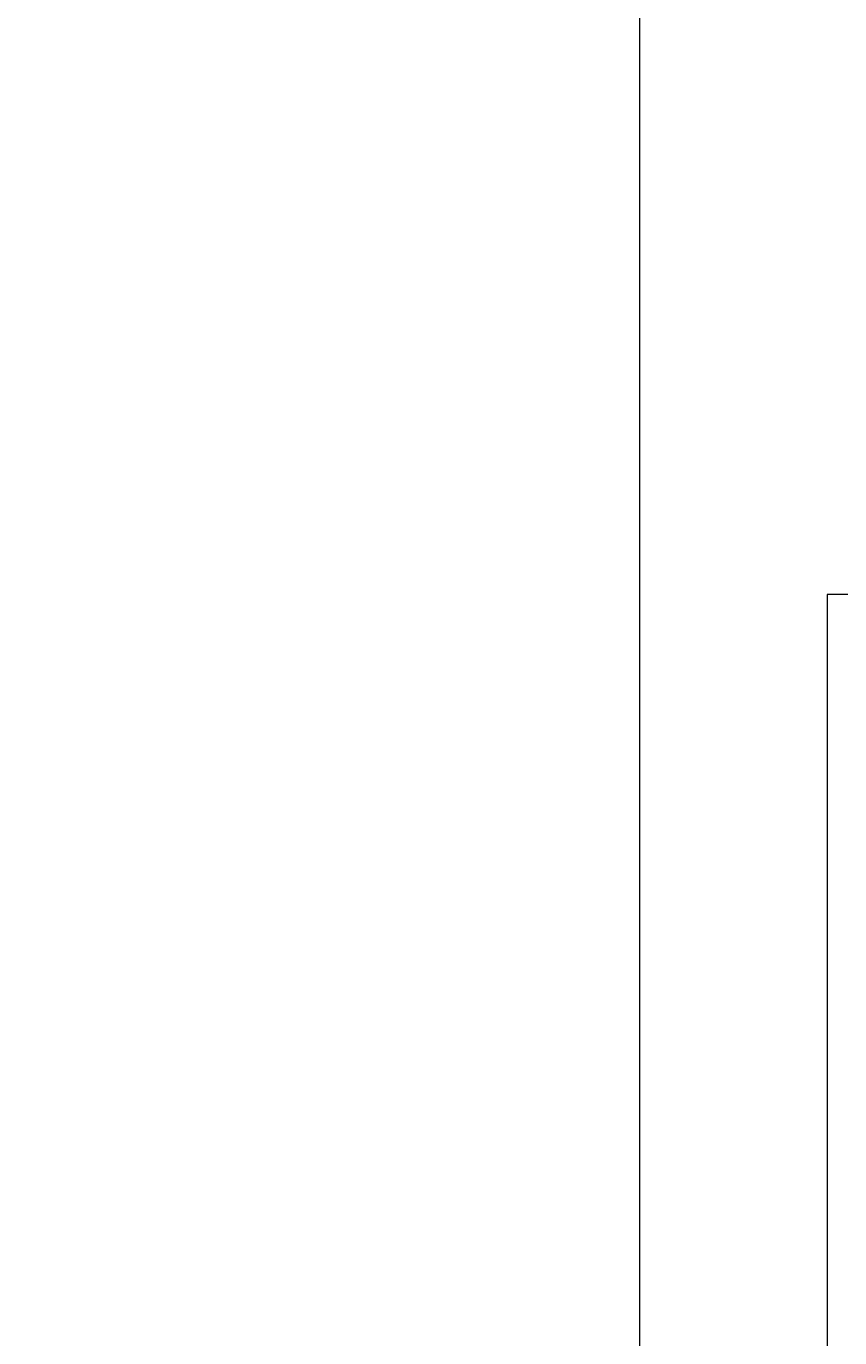
# Model space of a CAD drawing. Units: inches. Extents: x 1568 to 2529, y 2149 to 2897.
# Tile 6 of 16: x 1929 to 1944, y 2386 to 2410. Entities that reach past the tile are written whole.
import ezdxf

# ---------------------------------------------------------------- set-up
doc = ezdxf.new("R2010")
doc.units = ezdxf.units.IN
for name, color, linetype, lineweight in [('A-ANNO-DIMS', 2, 'Continuous', 18), ('A-EQPM', 8, 'Continuous', 18), ('A-FLOR-FIXT', 9, 'Continuous', 18)]:
    doc.layers.add(name, color=color, linetype=linetype, lineweight=lineweight)
doc.styles.get("Standard").update_dxf_attribs({"font": 'arial.ttf'})
doc.dimstyles.get("Standard").update_dxf_attribs({"dimtxt": 0.18, "dimasz": 0.18, "dimexe": 0.18, "dimexo": 0.0625, "dimgap": 0.09, "dimtad": 0, "dimtih": 1, "dimtoh": 1, "dimdec": 4, "dimzin": 0, "dimdsep": 46, "dimtxsty": 'Standard', "dimcen": 0.09, "dimadec": 0, "dimazin": 0, "dimtfac": 1, "dimtdec": 4, "dimtofl": 0, "dimtmove": 0, "dimatfit": 3, "dimfxl": 1, "dimtolj": 1, "dimtzin": 0, "dimarcsym": 0})

# ---------------------------------------------------------------- blocks, each defined once
blk = doc.blocks.new('*D32')
at = {"layer": 'A-ANNO-DIMS', "color": 0, "lineweight": -2, "transparency": 16777216}
for p, q in [((1964.551, 2792.469), (1964.551, 2165.502)), ((1904.551, 2753.401), (1904.551, 2165.502)), ((1904.731, 2165.682), (1934.332, 2165.682)), ((1964.371, 2165.682), (1934.77, 2165.682))]:
    blk.add_line(p, q, dxfattribs=at)
at = {"layer": 'A-ANNO-DIMS', "color": 0, "transparency": 16777216}
for points in [[(1904.731, 2165.712), (1904.731, 2165.652), (1904.551, 2165.682)], [(1964.371, 2165.712), (1964.371, 2165.652), (1964.551, 2165.682)]]:
    blk.add_solid(points, dxfattribs=at)
at = {"layer": 'Defpoints', "color": 0, "transparency": 16777216}
for p in [(1964.551, 2792.532), (1904.551, 2753.463), (1964.551, 2165.682)]:
    blk.add_point(p, dxfattribs=at)
at = {"layer": 'A-ANNO-DIMS', "color": 0, "transparency": 16777216, "insert": (1934.551, 2165.682), "char_height": 0.18, "attachment_point": 5}
blk.add_mtext('\\A1;60', dxfattribs=at)

msp = doc.modelspace()

# ---------------------------------------------------------------- linework, layer by layer
at = {"layer": 'A-EQPM'}
msp.add_lwpolyline([(1944.063, 2365.7088), (1961.4053, 2365.7088), (1961.4053, 2399.6535), (1944.063, 2399.6535)], close=True, dxfattribs=at)
at = {"layer": 'A-FLOR-FIXT'}
msp.add_line((1940.5509, 2471.532), (1940.5509, 2339.532), dxfattribs=at)

# ---------------------------------------------------------------- dimensions: what is measured, and where the dimension line sits
at = {"layer": 'A-ANNO-DIMS'}
dim = msp.add_linear_dim(base=(1964.5509, 2165.682), p1=(1904.5509, 2753.4635), p2=(1964.5509, 2792.532), dimstyle='Standard', override={"dimdec": 0, "dimlfac": 1, "dimrnd": 0, "dimzin": 0, "dimdsep": 46, "dimlunit": 2}, dxfattribs=at)
dim.commit()
dim.dimension.update_dxf_attribs({"geometry": '*D32', "text_midpoint": (1934.5509, 2165.682)})

doc.saveas('drawing.dxf')
